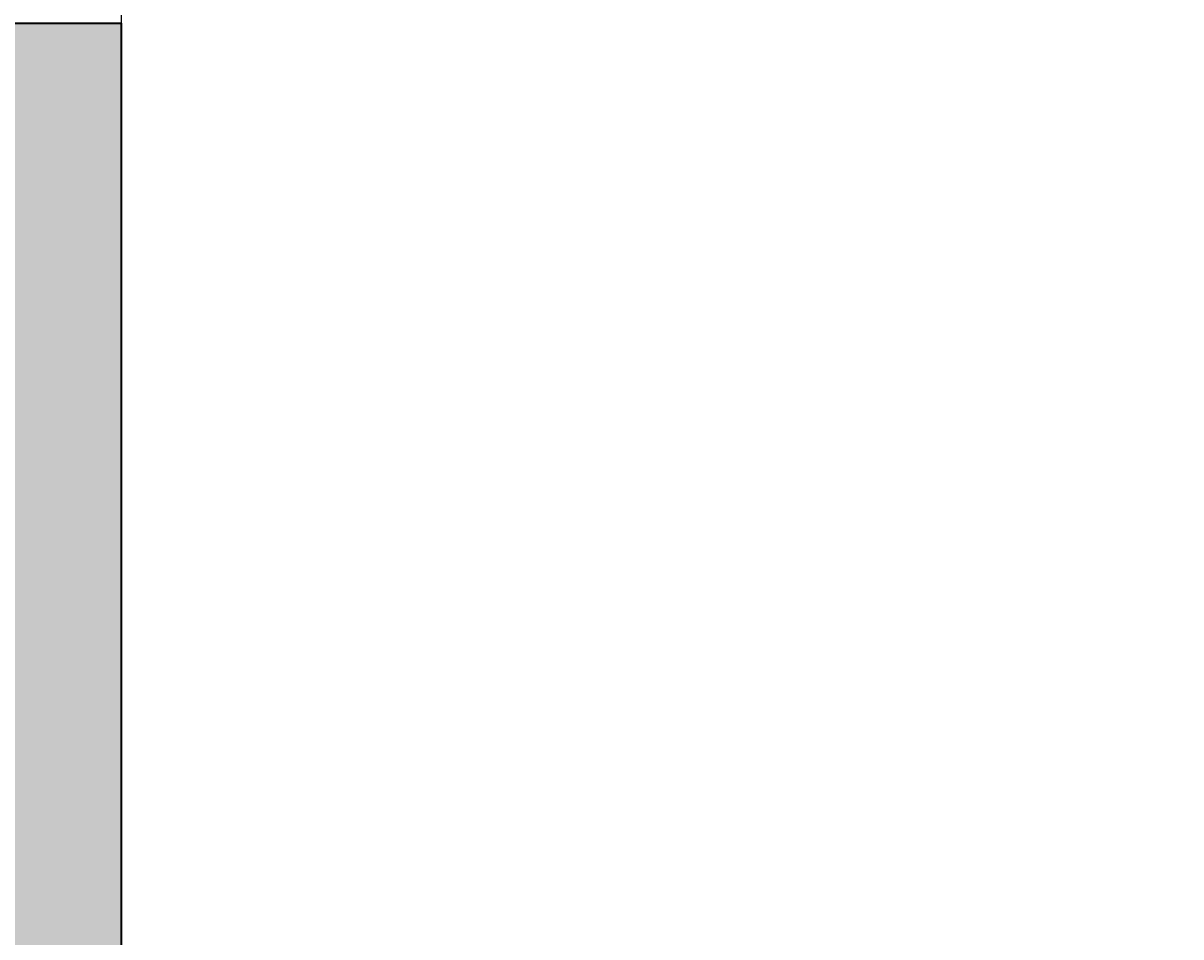
# Model space of a CAD drawing. Units: inches. Extents: x 1998 to 2588, y 1139 to 1977.
# Tile 81 of 134: x 2344 to 2370, y 1502 to 1523. Entities that reach past the tile are written whole.
import ezdxf

# ---------------------------------------------------------------- set-up
doc = ezdxf.new("R2010")
doc.units = ezdxf.units.IN
for name, color, linetype, lineweight in [('A-ANNO-DIMS', 2, 'Continuous', 18), ('A-WALL-PATT', 252, 'Continuous', 13), ('WALL', 200, 'Continuous', 35)]:
    doc.layers.add(name, color=color, linetype=linetype, lineweight=lineweight)
doc.styles.get("Standard").update_dxf_attribs({"font": 'arial.ttf'})
doc.dimstyles.get("Standard").update_dxf_attribs({"dimtxt": 0.18, "dimasz": 0.18, "dimexe": 0.18, "dimexo": 0.0625, "dimgap": 0.09, "dimtad": 0, "dimtih": 1, "dimtoh": 1, "dimdec": 4, "dimzin": 0, "dimdsep": 46, "dimtxsty": 'Standard', "dimcen": 0.09, "dimadec": 0, "dimazin": 0, "dimtfac": 1, "dimtdec": 4, "dimtofl": 0, "dimtmove": 0, "dimatfit": 3, "dimfxl": 1, "dimtolj": 1, "dimtzin": 0, "dimarcsym": 0})

# ---------------------------------------------------------------- blocks, each defined once
blk = doc.blocks.new('*D43')
at = {"layer": 'A-ANNO-DIMS', "color": 0, "lineweight": -2, "transparency": 16777216}
for p, q in [((2407.973, 1594.67), (2407.973, 1138.602)), ((2345.973, 1588.67), (2345.973, 1138.602)), ((2346.153, 1138.782), (2376.754, 1138.782)), ((2407.793, 1138.782), (2377.191, 1138.782))]:
    blk.add_line(p, q, dxfattribs=at)
at = {"layer": 'A-ANNO-DIMS', "color": 0, "transparency": 16777216}
for points in [[(2346.153, 1138.812), (2346.153, 1138.752), (2345.973, 1138.782)], [(2407.793, 1138.812), (2407.793, 1138.752), (2407.973, 1138.782)]]:
    blk.add_solid(points, dxfattribs=at)
at = {"layer": 'Defpoints', "color": 0, "transparency": 16777216}
for p in [(2407.973, 1594.732), (2345.973, 1588.732), (2407.973, 1138.782)]:
    blk.add_point(p, dxfattribs=at)
at = {"layer": 'A-ANNO-DIMS', "color": 0, "transparency": 16777216, "insert": (2376.973, 1138.782), "char_height": 0.18, "attachment_point": 5}
blk.add_mtext('\\A1;62', dxfattribs=at)

msp = doc.modelspace()

# ---------------------------------------------------------------- hatches: boundary and pattern name
at = {"layer": 'A-WALL-PATT'}
h = msp.add_hatch(color=256, dxfattribs=at)
h.dxf.hatch_style = 1
h.paths.add_polyline_path([(2222.9729, 1888.7324), (2099.4125, 1888.7324), (2099.4125, 1879.7324), (2222.9729, 1879.7324)])
h.paths.add_polyline_path([(2096.9729, 1868.3278), (2087.9729, 1868.3278), (2087.9729, 1775.637), (2096.9729, 1775.637)])
h.paths.add_polyline_path([(2227.4729, 1868.3278), (2222.9729, 1868.3278), (2222.9729, 1774.3318), (2227.4729, 1774.3318)])
h.paths.add_polyline_path([(2188.3019, 1759.7324), (2138.6074, 1759.7324), (2099.4125, 1759.7324), (2099.4125, 1755.2324), (2176.9729, 1755.2324), (2188.3019, 1755.2324)])
h.paths.add_polyline_path([(2087.9729, 1759.7324), (2059.4729, 1759.7324), (2059.4729, 1702.7324), (2087.9729, 1702.7324), (2087.9729, 1707.2324), (2063.9729, 1707.2324), (2063.9729, 1755.2324), (2087.9729, 1755.2324)])
h.paths.add_polyline_path([(2096.9729, 1755.2324), (2087.9729, 1755.2324), (2087.9729, 1707.2324), (2096.9729, 1707.2324)])
h.paths.add_polyline_path([(2187.0461, 1707.2324), (2105.9729, 1707.2324), (2096.9729, 1707.2324), (2087.9729, 1707.2324), (2087.9729, 1702.7324), (2105.9729, 1702.7324), (2114.9729, 1702.7324), (2187.0461, 1702.7324)])
h.paths.add_polyline_path([(2181.4729, 1719.2028), (2176.9729, 1719.2028), (2176.9729, 1707.2324), (2181.4729, 1707.2324)])
h.paths.add_polyline_path([(2216.0332, 1588.7324), (2114.9729, 1588.7324), (2105.9729, 1588.7324), (2105.9729, 1584.2324), (2216.0332, 1584.2324)])
h.paths.add_polyline_path([(2077.691, 1588.7324), (2061.4729, 1588.7324), (2061.4729, 1584.2324), (2077.691, 1584.2324)])
h.paths.add_polyline_path([(2105.9729, 1588.7324), (2098.0956, 1588.7324), (2098.0956, 1584.2324), (2105.9729, 1584.2324)])
h.paths.add_polyline_path([(2114.9729, 1596.2642), (2110.1012, 1596.2642), (2105.9729, 1596.2642), (2105.9729, 1588.7324), (2114.9729, 1588.7324)])
h.paths.add_polyline_path([(2114.9729, 1584.2324), (2105.9729, 1584.2324), (2105.9729, 1580.249), (2110.1012, 1580.249), (2114.9729, 1580.249)])
h.paths.add_polyline_path([(2114.9729, 1547.7716), (2110.1012, 1547.7716, -0.0318759), (2105.9729, 1548.035), (2105.9729, 1470.2324), (2108.3775, 1470.2324), (2108.3775, 1465.7324), (2186.2943, 1465.7324), (2186.2943, 1470.2324), (2114.9729, 1470.2324)])
h.paths.add_polyline_path([(2227.4729, 1584.2324), (2222.9729, 1584.2324), (2222.9729, 1486.137), (2227.4729, 1486.137)])
h.paths.add_polyline_path([(2295.4138, 1593.2324), (2227.4729, 1593.2324), (2227.4729, 1588.7324), (2295.4138, 1588.7324), (2295.4138, 1591.8729)])
h.paths.add_polyline_path([(2345.9729, 1627.1165), (2341.4729, 1627.1165), (2341.4729, 1593.2324), (2337.2869, 1593.2324), (2337.2869, 1591.8729), (2337.2869, 1588.7324), (2345.9729, 1588.7324)])
h.paths.add_polyline_path([(2291.9729, 1588.7324), (2287.4729, 1588.7324), (2287.4729, 1522.7324), (2291.9729, 1522.7324)])
h.paths.add_polyline_path([(2291.9729, 1522.7324), (2287.4729, 1522.7324), (2227.4729, 1522.7324), (2227.4729, 1518.2324), (2291.9729, 1518.2324)])
h.paths.add_polyline_path([(2295.7347, 1519.5919), (2295.7347, 1522.7324), (2291.9729, 1522.7324), (2291.9729, 1518.2324), (2295.7347, 1518.2324)])
h.paths.add_polyline_path([(2345.9729, 1522.7324), (2337.6078, 1522.7324), (2337.6078, 1519.5919), (2337.6078, 1518.2324), (2341.4729, 1518.2324), (2341.4729, 1488.5616), (2345.9729, 1488.5616)])
h.paths.add_polyline_path([(2345.9729, 1468.1569), (2341.4729, 1468.1569), (2341.4729, 1374.2324), (2227.4729, 1374.2324), (2227.4729, 1369.7324), (2345.9729, 1369.7324)])
h.paths.add_polyline_path([(2345.9729, 1369.7324), (2341.4729, 1369.7324), (2341.4729, 1362.2324), (2345.9729, 1362.2324)])
h.paths.add_polyline_path([(2345.9729, 1317.7324), (2345.9729, 1322.2324), (2341.4729, 1322.2324), (2341.4729, 1285.137), (2345.9729, 1285.137)], flags=17)
h.paths.add_polyline_path([(2356.2096, 1322.2324), (2345.9729, 1322.2324), (2345.9729, 1317.7324), (2356.2096, 1317.7324), (2356.2096, 1319.3088)], flags=17)
h.paths.add_polyline_path([(2393.9729, 1322.2324), (2375.6999, 1322.2324), (2375.6999, 1319.3088, -0.0202458), (2375.636, 1317.7324), (2393.9729, 1317.7324)], flags=17)
h.paths.add_polyline_path([(2398.4729, 1322.2324), (2393.9729, 1322.2324), (2393.9729, 1317.7324), (2393.9729, 1237.7324), (2345.9729, 1237.7324), (2345.9729, 1264.7324), (2341.4729, 1264.7324), (2341.4729, 1228.7324), (2393.9729, 1228.7324), (2482.7412, 1228.7324), (2482.7412, 1237.7324), (2398.4729, 1237.7324), (2398.4729, 1297.1029)])
h.paths.add_polyline_path([(2398.4729, 1362.2324), (2393.9729, 1362.2324), (2393.9729, 1357.7324), (2398.4729, 1357.7324)])
h.paths.add_polyline_path([(2345.9729, 1329.7549), (2341.4729, 1329.7549), (2341.4729, 1322.2324), (2345.9729, 1322.2324)])

# ---------------------------------------------------------------- linework, layer by layer
at = {"layer": 'WALL'}
for p, q in [((2337.6078, 1522.7324), (2345.9729, 1522.7324)), ((2345.9729, 1522.7324), (2345.9729, 1369.7324)), ((2345.9729, 1522.7324), (2345.9729, 1480.7324))]:
    msp.add_line(p, q, dxfattribs=at)

# ---------------------------------------------------------------- dimensions: what is measured, and where the dimension line sits
at = {"layer": 'A-ANNO-DIMS'}
dim = msp.add_linear_dim(base=(2407.9729, 1138.7824), p1=(2345.9729, 1588.7324), p2=(2407.9729, 1594.7324), dimstyle='Standard', override={"dimdec": 0, "dimlfac": 1, "dimrnd": 0, "dimzin": 0, "dimdsep": 46, "dimlunit": 2}, dxfattribs=at)
dim.commit()
dim.dimension.update_dxf_attribs({"geometry": '*D43', "text_midpoint": (2376.9729, 1138.7824)})

doc.saveas('drawing.dxf')
